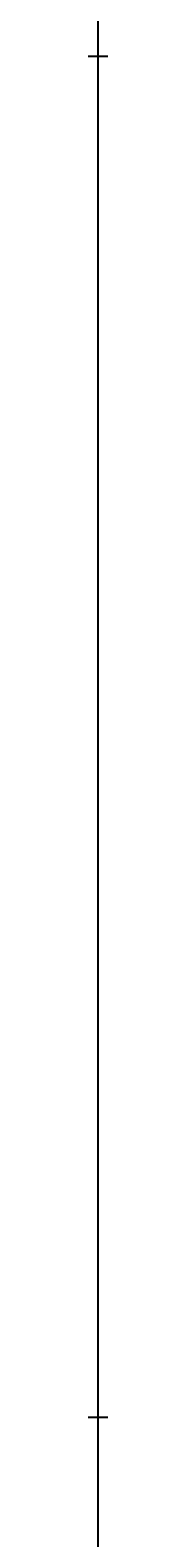
# Model space of a CAD drawing. Units: inches. Extents: x 35362 to 73946, y 43607 to 67532.
# Tile 41 of 134: x 48373 to 48374, y 46091 to 46564. Entities that reach past the tile are written whole.
import ezdxf

# ---------------------------------------------------------------- set-up
doc = ezdxf.new("R2010")
doc.units = ezdxf.units.IN
doc.header["$MEASUREMENT"] = 0
doc.layers.add('A-ANNO-DIMS', color=2, linetype='Continuous', lineweight=18)
doc.styles.get("Standard").update_dxf_attribs({"font": 'arial.ttf'})
doc.dimstyles.get("Standard").update_dxf_attribs({"dimtxt": 0.18, "dimasz": 0.18, "dimexe": 0.18, "dimexo": 0.0625, "dimgap": 0.09, "dimtad": 0, "dimtih": 1, "dimtoh": 1, "dimdec": 4, "dimzin": 0, "dimdsep": 46, "dimtxsty": 'Standard', "dimcen": 0.09, "dimadec": 0, "dimazin": 0, "dimtfac": 1, "dimtdec": 4, "dimtofl": 0, "dimtmove": 0, "dimatfit": 3, "dimfxl": 1, "dimtolj": 1, "dimtzin": 0, "dimarcsym": 0})

# ---------------------------------------------------------------- blocks, each defined once
blk = doc.blocks.new('*D5')
at = {"layer": 'A-ANNO-DIMS', "color": 0, "lineweight": -2, "transparency": 16777216}
for p, q in [((37121.95, 46919.32), (37121.95, 43606.68)), ((69871.5, 45449.83), (69871.5, 43606.68)), ((37122.13, 43606.86), (53496.29, 43606.86)), ((69871.32, 43606.86), (53497.15, 43606.86))]:
    blk.add_line(p, q, dxfattribs=at)
at = {"layer": 'A-ANNO-DIMS', "color": 0, "transparency": 16777216}
for points in [[(37122.13, 43606.89), (37122.13, 43606.83), (37121.95, 43606.86)], [(69871.32, 43606.89), (69871.32, 43606.83), (69871.5, 43606.86)]]:
    blk.add_solid(points, dxfattribs=at)
at = {"layer": 'Defpoints', "color": 0, "transparency": 16777216}
for p in [(37121.95, 46919.38), (69871.5, 45449.89), (69871.5, 43606.86)]:
    blk.add_point(p, dxfattribs=at)
at = {"layer": 'A-ANNO-DIMS', "color": 0, "transparency": 16777216, "insert": (53496.72, 43606.86), "char_height": 0.18, "attachment_point": 5}
blk.add_mtext('\\A1;32750', dxfattribs=at)
blk = doc.blocks.new('*D11')
at = {"layer": 'A-ANNO-DIMS', "color": 0, "lineweight": -2, "transparency": 16777216}
for p, q in [((47978.66, 56028.77), (47978.66, 43606.68)), ((53109.76, 56028.77), (53109.76, 43606.68)), ((47978.84, 43606.86), (50543.87, 43606.86)), ((53109.58, 43606.86), (50544.55, 43606.86))]:
    blk.add_line(p, q, dxfattribs=at)
at = {"layer": 'A-ANNO-DIMS', "color": 0, "transparency": 16777216}
for points in [[(47978.84, 43606.89), (47978.84, 43606.83), (47978.66, 43606.86)], [(53109.58, 43606.89), (53109.58, 43606.83), (53109.76, 43606.86)]]:
    blk.add_solid(points, dxfattribs=at)
at = {"layer": 'Defpoints', "color": 0, "transparency": 16777216}
for p in [(47978.66, 56028.84), (53109.76, 56028.84), (53109.76, 43606.86)]:
    blk.add_point(p, dxfattribs=at)
at = {"layer": 'A-ANNO-DIMS', "color": 0, "transparency": 16777216, "insert": (50544.21, 43606.86), "char_height": 0.18, "attachment_point": 5}
blk.add_mtext('\\A1;5131', dxfattribs=at)
blk = doc.blocks.new('*D13')
at = {"layer": 'A-ANNO-DIMS', "color": 0, "lineweight": -2, "transparency": 16777216}
for p, q in [((48373.49, 51694.02), (48373.49, 43606.68)), ((51029.04, 51694.02), (51029.04, 43606.68)), ((48373.67, 43606.86), (49700.8, 43606.86)), ((51028.86, 43606.86), (49701.73, 43606.86))]:
    blk.add_line(p, q, dxfattribs=at)
at = {"layer": 'A-ANNO-DIMS', "color": 0, "transparency": 16777216}
for points in [[(48373.67, 43606.89), (48373.67, 43606.83), (48373.49, 43606.86)], [(51028.86, 43606.89), (51028.86, 43606.83), (51029.04, 43606.86)]]:
    blk.add_solid(points, dxfattribs=at)
at = {"layer": 'Defpoints', "color": 0, "transparency": 16777216}
for p in [(48373.49, 51694.09), (51029.04, 51694.09), (51029.04, 43606.86)]:
    blk.add_point(p, dxfattribs=at)
at = {"layer": 'A-ANNO-DIMS', "color": 0, "transparency": 16777216, "insert": (49701.27, 43606.86), "char_height": 0.18, "attachment_point": 5}
blk.add_mtext('\\A1;2655.6', dxfattribs=at)
blk = doc.blocks.new('*D67')
at = {"layer": 'A-ANNO-DIMS', "color": 0, "lineweight": -2, "transparency": 16777216}
for p, q in [((56873.54, 53351.53), (35361.77, 53351.53)), ((35361.95, 53351.35), (35361.95, 49400.89)), ((35361.95, 45450.07), (35361.95, 49400.53)), ((53793.58, 45449.89), (35361.77, 45449.89))]:
    blk.add_line(p, q, dxfattribs=at)
at = {"layer": 'A-ANNO-DIMS', "color": 0, "transparency": 16777216}
for points in [[(35361.92, 53351.35), (35361.98, 53351.35), (35361.95, 53351.53)], [(35361.92, 45450.07), (35361.98, 45450.07), (35361.95, 45449.89)]]:
    blk.add_solid(points, dxfattribs=at)
at = {"layer": 'Defpoints', "color": 0, "transparency": 16777216}
for p in [(35361.95, 53351.53), (56873.6, 53351.53), (53793.64, 45449.89)]:
    blk.add_point(p, dxfattribs=at)
at = {"layer": 'A-ANNO-DIMS', "color": 0, "transparency": 16777216, "insert": (35361.95, 49400.71), "char_height": 0.18, "attachment_point": 5}
blk.add_mtext('\\A1;7901.6', dxfattribs=at)
blk = doc.blocks.new('*D76')
at = {"layer": 'A-ANNO-DIMS', "color": 0, "lineweight": -2, "transparency": 16777216}
for p, q in [((54052.84, 46555.29), (35361.77, 46555.29)), ((35361.95, 46555.11), (35361.95, 46342.27)), ((35361.95, 46129.06), (35361.95, 46341.9)), ((53793.58, 46128.88), (35361.77, 46128.88))]:
    blk.add_line(p, q, dxfattribs=at)
at = {"layer": 'A-ANNO-DIMS', "color": 0, "transparency": 16777216}
for points in [[(35361.92, 46555.11), (35361.98, 46555.11), (35361.95, 46555.29)], [(35361.92, 46129.06), (35361.98, 46129.06), (35361.95, 46128.88)]]:
    blk.add_solid(points, dxfattribs=at)
at = {"layer": 'Defpoints', "color": 0, "transparency": 16777216}
for p in [(35361.95, 46555.29), (54052.9, 46555.29), (53793.64, 46128.88)]:
    blk.add_point(p, dxfattribs=at)
at = {"layer": 'A-ANNO-DIMS', "color": 0, "transparency": 16777216, "insert": (35361.95, 46342.09), "char_height": 0.18, "attachment_point": 5}
blk.add_mtext('\\A1;426.4', dxfattribs=at)
blk = doc.blocks.new('*D90')
at = {"layer": 'A-ANNO-DIMS', "color": 0, "lineweight": -2, "transparency": 16777216}
for p, q in [((53707.72, 47291.29), (35361.77, 47291.29)), ((35361.95, 47291.11), (35361.95, 46710.26)), ((35361.95, 46129.06), (35361.95, 46709.9)), ((53793.58, 46128.88), (35361.77, 46128.88))]:
    blk.add_line(p, q, dxfattribs=at)
at = {"layer": 'A-ANNO-DIMS', "color": 0, "transparency": 16777216}
for points in [[(35361.92, 47291.11), (35361.98, 47291.11), (35361.95, 47291.29)], [(35361.92, 46129.06), (35361.98, 46129.06), (35361.95, 46128.88)]]:
    blk.add_solid(points, dxfattribs=at)
at = {"layer": 'Defpoints', "color": 0, "transparency": 16777216}
for p in [(53707.78, 47291.29), (35361.95, 46128.88), (53793.64, 46128.88)]:
    blk.add_point(p, dxfattribs=at)
at = {"layer": 'A-ANNO-DIMS', "color": 0, "transparency": 16777216, "insert": (35361.95, 46710.08), "char_height": 0.18, "attachment_point": 5}
blk.add_mtext('\\A1;1162.4', dxfattribs=at)

msp = doc.modelspace()

# ---------------------------------------------------------------- dimensions: what is measured, and where the dimension line sits
at = {"layer": 'A-ANNO-DIMS'}
for base, p1, p2, override, picture, middle in [((53109.76, 43606.859), (47978.665, 56028.836), (53109.76, 56028.836), {"dimdec": 0, "dimlfac": 1, "dimrnd": 0, "dimzin": 0, "dimdsep": 46, "dimlunit": 2}, '*D11', (50544.212, 43606.859)), ((51029.043, 43606.859), (48373.492, 51694.087), (51029.043, 51694.087), {"dimdec": 1, "dimlfac": 1, "dimrnd": 0, "dimzin": 0, "dimdsep": 46, "dimlunit": 2}, '*D13', (49701.267, 43606.859)), ((69871.496, 43606.859), (37121.949, 46919.381), (69871.496, 45449.894), {"dimdec": 0, "dimlfac": 1, "dimrnd": 0, "dimzin": 0, "dimdsep": 46, "dimlunit": 2}, '*D5', (53496.723, 43606.859))]:
    dim = msp.add_linear_dim(base=base, p1=p1, p2=p2, dimstyle='Standard', override=override, dxfattribs=at)
    dim.commit()
    dim.dimension.update_dxf_attribs({"geometry": picture, "text_midpoint": middle})
for base, p1, p2, picture, middle in [((35361.949, 53351.529), (53793.638, 45449.894), (56873.602, 53351.529), '*D67', (35361.949, 49400.712)), ((35361.949, 46128.878), (53707.781, 47291.285), (53793.638, 46128.878), '*D90', (35361.949, 46710.081)), ((35361.949, 46555.293), (53793.638, 46128.878), (54052.899, 46555.293), '*D76', (35361.949, 46342.086))]:
    dim = msp.add_linear_dim(base=base, p1=p1, p2=p2, angle=90, dimstyle='Standard', override={"dimdec": 1, "dimlfac": 1, "dimrnd": 0, "dimzin": 0, "dimdsep": 46, "dimlunit": 2}, dxfattribs=at)
    dim.commit()
    dim.dimension.update_dxf_attribs({"geometry": picture, "text_midpoint": middle})

doc.saveas('drawing.dxf')
